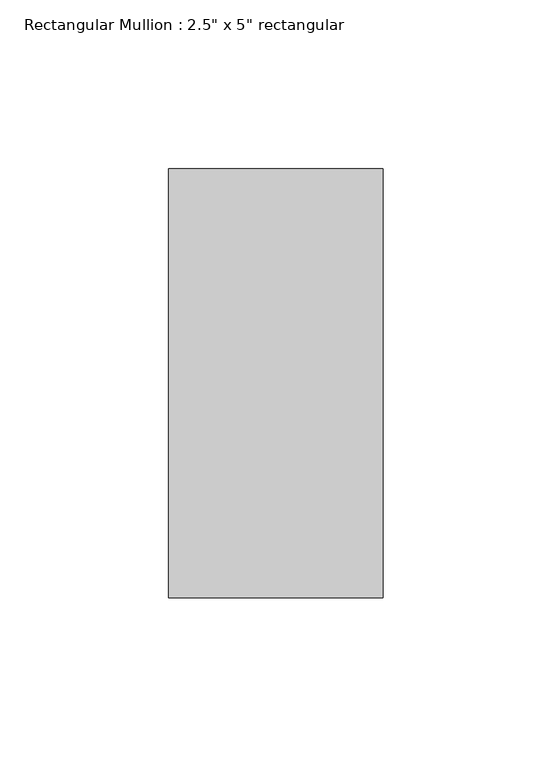
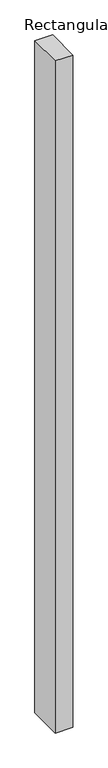
"""IFC4 building model written with IfcOpenShell, lengths in millimetres: member geometry."""

from ifc_helpers import new_model, si_unit, frame, origin, place, context, project, spatial, polyline, outline, extrude, source, transform, mapped, element, save


def member_6a413f91(model_context):
    return source(origin(), model_context, "Body", "SweptSolid", [
        extrude(outline(polyline([(0.0, 63.5), (0.0, -63.5), (-63.5, -63.5), (-63.5, 63.5), (0.0, 63.5)])), frame((0.0, 0.0, -2560.9471371), z_axis=(0.0, 0.0, 1.0), x_axis=(1.0, 0.0, 0.0)), (0.0, 0.0, 1.0), 2560.9471371),
    ])


if __name__ == "__main__":
    model = new_model("IFC4")
    model_context = context("Model", 3, world=origin())
    ifc_project = project(units=[si_unit("LENGTHUNIT", "METRE", prefix="MILLI")], contexts=[model_context])
    site = spatial("IfcSite", under=ifc_project)
    building = spatial("IfcBuilding", under=site)
    placement = place(None, origin())
    member_shape = member_6a413f91(model_context)
    element("IfcMember", 1, ObjectType="Rectangular Mullion : 2.5\" x 5\" rectangular", at=placement, inside=building, context=model_context, shape_type="MappedRepresentation", body=[
        mapped(member_shape, transform((0.0, 0.0, 0.0), x_axis=(1.0, 0.0, 0.0), y_axis=(0.0, 1.0, 0.0), z_axis=(0.0, 0.0, 1.0))),
    ])
    save(model, "model.ifc")

# Revit data of these elements
# Type "Rectangular Mullion : 2.5\" x 5\" rectangular"
#   built-in parameter 1007304 = 0.416667 (stored number, unit not read)
#   built-in parameter 1007301 = 0.104167 (stored number, unit not read)
#   built-in parameter 1007300 = 0.104167 (stored number, unit not read)
# Element 1 (IfcMember, "Rectangular Mullion : 2.5\" x 5\" rectangular")
#   Materials on its faces: "Aluminum"
# Materials
#   "Aluminum": class "Metal", colour RGB 247 247 247, transparency 0, Description = "Aluminum 6061", Cost = 0
